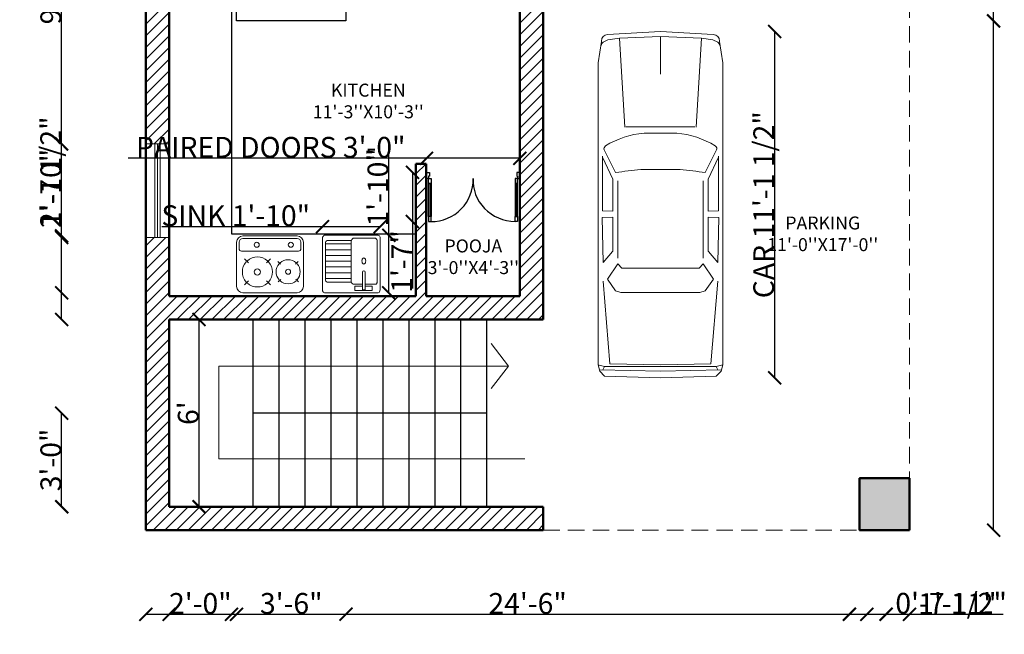
# Model space of a CAD drawing. Units: inches. Extents: x 1385 to 1778, y 1343 to 2100.
# Tile 1 of 6: x 1385 to 1764, y 1343 to 1579. Entities that reach past the tile are written whole.
import ezdxf

# ---------------------------------------------------------------- set-up
doc = ezdxf.new("R2010")
doc.units = ezdxf.units.IN
doc.linetypes.add('HIDDEN', pattern=[9.525, 6.35, -3.175])
for name, color, linetype, lineweight in [('A-ANNO-DIMS', 2, 'Continuous', 18), ('A-ANNO-SYMB', 50, 'Continuous', 18), ('A-AREA-IDEN', 7, 'Continuous', 25), ('A-COLS', 10, 'Continuous', 50), ('A-COLS-PATT', 10, 'Continuous', 13), ('A-EQPM', 9, 'Continuous', 18), ('A-FLOR-FIXT', 9, 'Continuous', 18), ('A-SITE-VEHI', 8, 'Continuous', 18), ('A-WALL-HIDN', 7, 'HIDDEN', 18), ('A-WALL-PATT', 8, 'Continuous', 13), ('Door', 150, 'Continuous', 25), ('Kitchen', 142, 'Continuous', 25), ('Steps', 50, 'Continuous', 25), ('Wall', 7, 'Continuous', 50), ('Windows', 140, 'Continuous', 18)]:
    doc.layers.add(name, color=color, linetype=linetype, lineweight=lineweight)
doc.layers.add('A-Glaz', color=92, linetype='Continuous')
doc.styles.get("Standard").update_dxf_attribs({"font": 'arial.ttf'})
doc.dimstyles.get("Standard").update_dxf_attribs({"dimtxt": 8, "dimasz": 5, "dimexe": 0.18, "dimexo": 0.0625, "dimgap": 0.09, "dimtad": 1, "dimdec": 1, "dimzin": 0, "dimdsep": 46, "dimlunit": 4, "dimtxsty": 'Standard', "dimblk": 'ARCHTICK', "dimcen": 0.09, "dimse1": 1, "dimse2": 1, "dimadec": 0, "dimazin": 0, "dimtfac": 1, "dimtdec": 1, "dimtofl": 0, "dimtmove": 0, "dimatfit": 3, "dimfxl": 1, "dimtolj": 1, "dimtzin": 0, "dimarcsym": 0})

# ---------------------------------------------------------------- blocks, each defined once
blk = doc.blocks.new('A$C13CE0A17')
at = {"layer": 'A-Glaz'}
for p, q in [((0.01, 0.61), (0.01, 0.08)), ((0.03, 0.08), (0.03, 0.61))]:
    blk.add_line(p, q, dxfattribs=at)
blk.add_lwpolyline([(1.4, 0.08), (1.4, 0.61), (1.42, 0.61), (1.42, 0.08)], close=True, dxfattribs=at)
at = {"layer": 'Door'}
for p, q in [((0, 0.61), (0, 0.69)), ((0, 0.69), (0.04, 0.69)), ((0.04, 0.69), (0.04, 0.61)), ((0, 0.61), (0, 0.08)), ((0.04, 0.61), (0, 0.61)), ((0.04, 0.61), (0, 0.61)), ((0.03, 0.61), (0.01, 0.61)), ((0.04, 0.08), (0.04, 0.61)), ((-0.035, 0), (-0.035, -0.1)), ((0, 0), (-0.035, 0)), ((0, 0.08), (0, 0)), ((0.04, 0.08), (0, 0.08)), ((0, 0.08), (0.04, 0.08)), ((0, 0), (0.04, 0)), ((0, -0.04), (0, 0)), ((0.01, 0.08), (0.03, 0.08)), ((0.04, 0), (0.04, 0.08)), ((-0.035, -0.1), (0.015, -0.1)), ((0.015, -0.04), (0, -0.04)), ((0.015, -0.05), (0.015, -0.04)), ((0.015, -0.1), (0.015, -0.05))]:
    blk.add_line(p, q, dxfattribs=at)
for points in [[(1.39, 0.69), (1.39, 0.61), (1.43, 0.61), (1.43, 0.69)], [(1.39, 0.08), (1.39, 0.61), (1.43, 0.61), (1.43, 0.08)], [(1.39, 0), (1.39, 0.08), (1.43, 0.08), (1.43, 0)], [(1.43, 0), (1.465, 0), (1.465, -0.1), (1.415, -0.1), (1.415, -0.05), (1.415, -0.04), (1.43, -0.04)]]:
    blk.add_lwpolyline(points, close=True, dxfattribs=at)
blk.add_arc((1.387, 0.017), 0.673, 89.7657, 181.4438, dxfattribs=at)
blk.add_ellipse((0.039, 0.051), major_axis=(0.667, -0.122), ratio=0.940794, start_param=0.11153, end_param=1.73917, dxfattribs=at)
blk = doc.blocks.new('02PCAR12')
at = {"color": 0, "linetype": 'ByBlock'}
for p, q in [((-207, 37), (-210, 34)), ((-203, 38), (-207, 37)), ((-206, 37), (-207, 0)), ((-203, 38.08), (-204, 34.08)), ((-19, 38), (-203, 38)), ((-6, 36), (-19, 38)), ((-210, 34), (-211, 0)), ((-204, 34.08), (-206, 35.08)), ((-204, -34), (-204, 34)), ((-202.36, 30.78), (-203, 0)), ((-202.36, 30.78), (-152, 35)), ((-150.83, 32.3), (-157.9, 27.3)), ((-141.48, 25.99), (-150.83, 32.3)), ((-113.23, 35.5), (-140.79, 34.89)), ((-140.79, 34.89), (-133.96, 29.23)), ((-113, 29), (-113.23, 35.5)), ((-109.42, 29.02), (-109.19, 35.33)), ((-109.19, 35.33), (-75.91, 35.3)), ((-76.45, 35.3), (-90, 29)), ((-72.15, 34.24), (-85.91, 27.37)), ((-5, 32), (-6.45, 34.89)), ((-5, 32), (-4, 25)), ((0, 0), (-1.8, 32.21)), ((-157.9, 27.3), (-158.93, 24.08)), ((-158.93, 24.08), (-158.93, -24)), ((-141.48, 25.99), (-144.24, 23.52)), ((-91, 26), (-138, 26)), ((-134, 29), (-113, 29)), ((-90, 29), (-109.42, 29.02)), ((-58.25, 21.76), (-4, 25)), ((-4, 25), (-3, 0)), ((-144.24, 23.52), (-144.24, 0)), ((-58, 0), (-58, 21)), ((-84, -12), (-84, 12)), ((-62, 10), (-62, 0)), ((-210, -34), (-211, 0)), ((-206, -37), (-207, 0)), ((-202.36, -30.78), (-203, 0)), ((-144.24, -23.52), (-144.24, 0)), ((-62, -10), (-62, 0)), ((-58, 0), (-58, -21)), ((-3, 0), (-26, 0)), ((-4, -25), (-3, 0)), ((0, 0), (-1.8, -32.21)), ((-141.48, -25.99), (-144.24, -23.52)), ((-58.25, -21.76), (-4, -25)), ((-157.9, -27.3), (-158.93, -24.08)), ((-150.83, -32.3), (-157.9, -27.3)), ((-141.48, -25.99), (-150.83, -32.3)), ((-140.79, -34.89), (-133.96, -29.23)), ((-91, -26), (-138, -26)), ((-134, -29), (-113, -29)), ((-113, -29), (-113.23, -35.5)), ((-90, -29), (-109.42, -29.02)), ((-109.42, -29.02), (-109.19, -35.33)), ((-76.45, -35.3), (-90, -29)), ((-72.15, -34.24), (-85.91, -27.37)), ((-5, -32), (-4, -25)), ((-207, -37), (-210, -34)), ((-204, -34), (-206, -35)), ((-203, -38), (-204, -34)), ((-202.36, -30.69), (-152, -34.92)), ((-113.23, -35.5), (-140.79, -34.89)), ((-109.19, -35.33), (-75.91, -35.3)), ((-6, -36), (-19, -38)), ((-5, -32), (-6.45, -34.89)), ((-203, -38), (-207, -37)), ((-19, -38), (-203, -38))]:
    blk.add_line(p, q, dxfattribs=at)
for centre, radius, start, end in [((-71.36, 32.4), 2, 31.5638, 113.12574), ((-115.33, 5.39), 53.61, 4.93792, 31.5638), ((-8.24, 34), 2, 26.56505, 90), ((-5.8, 32), 4, 3.01279, 90), ((-461.05, -27.14), 379.08, 5.92644, 8.26698), ((-461.05, 27.14), 379.08, 351.73302, 354.07356), ((-115.33, -5.39), 53.61, 328.4362, 355.06208), ((-71.36, -32.4), 2, 246.87426, 328.4362), ((-8.24, -34), 2, 270, 333.43495), ((-5.8, -32), 4, 270, 356.98721)]:
    blk.add_arc(centre, radius, start, end, dxfattribs=at)
blk = doc.blocks.new('S_SINK12')
for p, q in [((0.25, 0.45), (0.25, 0)), ((0.35, 0.45), (0.35, 0)), ((0.45, 0.45), (0.45, 0)), ((0.55, 0.45), (0.55, 0)), ((0.65, 0.45), (0.65, 0)), ((0.75, 0.45), (0.75, 0)), ((0.85, 0.45), (0.85, 0))]:
    blk.add_line(p, q)
for points in [[(0, -0.469), (0, 0.469, -0.310961), (0.05, 0.5), (0.95, 0.5, -0.310466), (1, 0.469), (1, -0.469, -0.414214), (0.969, -0.5), (0.05, -0.5, -0.309971)], [(0.052, -0.195), (0.052, -0.242), (0.362, -0.242, 1), (0.362, -0.195)], [(0.5, -0.217), (0.503, -0.229, 0.107136), (0.516, -0.241, 0.076468), (0.534, -0.249), (0.554, -0.251), (0.575, -0.248, 0.076468), (0.592, -0.241, 0.107136), (0.604, -0.229), (0.608, -0.217), (0.604, -0.205, 0.107136), (0.592, -0.193, 0.076468), (0.575, -0.186), (0.554, -0.183), (0.532, -0.186, 0.076468), (0.516, -0.193, 0.107136), (0.503, -0.205)]]:
    blk.add_lwpolyline(points, format="xyb", close=True)
for points in [[(0.185, -0.001), (0.185, 0.419, -0.310466), (0.235, 0.45), (0.862, 0.45, -0.310466), (0.912, 0.419), (0.912, 0, -0.310466)], [(0.15, -0.195), (0.15, -0.031, -0.310466), (0.2, 0), (0.9, 0, -0.310466), (0.95, -0.031), (0.95, -0.419, -0.310466), (0.9, -0.45), (0.2, -0.45), (0.18, -0.448, -0.071009), (0.165, -0.442, -0.106323), (0.153, -0.432), (0.15, -0.422), (0.151, -0.419)]]:
    blk.add_lwpolyline(points, format="xyb")
for points in [[(0.114, -0.242), (0.114, -0.364), (0.039, -0.364), (0.039, -0.064), (0.114, -0.064), (0.114, -0.195)], [(0.15, -0.419), (0.15, -0.242)]]:
    blk.add_lwpolyline(points)
blk = doc.blocks.new('_ArchTick')
at = {"color": 0, "linetype": 'ByBlock', "const_width": 0.15}
blk.add_lwpolyline([(-0.5, -0.5), (0.5, 0.5)], dxfattribs=at)
blk = doc.blocks.new('*D12')
at = {"layer": 'A-ANNO-DIMS', "color": 0, "lineweight": -2, "transparency": 16777216}
blk.add_line((1454.26, 1391.73), (1454.26, 1463.73), dxfattribs=at)
at = {"layer": 'Defpoints', "color": 0, "transparency": 16777216}
for p in [(1442.77, 1463.73), (1454.26, 1463.73), (1442.77, 1391.73)]:
    blk.add_point(p, dxfattribs=at)
at = {"layer": 'A-ANNO-DIMS', "color": 0, "lineweight": -2, "transparency": 16777216, "xscale": 5, "yscale": 5, "zscale": 5}
for p, rotation in [((1454.26, 1463.73), 90), ((1454.26, 1391.73), 270)]:
    blk.add_blockref('_ArchTick', p, dxfattribs=dict(at, rotation=rotation))
at = {"layer": 'A-ANNO-DIMS', "color": 0, "transparency": 16777216, "insert": (1450.09, 1427.73), "char_height": 8, "attachment_point": 5, "rotation": 90}
blk.add_mtext("\\A1;6'", dxfattribs=at)
blk = doc.blocks.new('WINDOW-GLAZING-36IN')
for p, q in [((0, 0), (0, 36)), ((1, 0), (1, 36)), ((2, 0), (2, 36))]:
    blk.add_line(p, q)
blk = doc.blocks.new('*D25')
at = {"layer": 'A-ANNO-DIMS', "color": 0, "lineweight": -2, "transparency": 16777216}
for p, q in [((1541.8, 1525.8), (1426.95, 1525.8)), ((1577.76, 1525.8), (1541.8, 1525.8))]:
    blk.add_line(p, q, dxfattribs=at)
at = {"layer": 'Defpoints', "color": 0, "transparency": 16777216}
for p in [(1541.8, 1525.8), (1541.8, 1520.41), (1577.76, 1520.41)]:
    blk.add_point(p, dxfattribs=at)
at = {"layer": 'A-ANNO-DIMS', "color": 0, "lineweight": -2, "transparency": 16777216, "xscale": 5, "yscale": 5, "zscale": 5, "rotation": 180}
blk.add_blockref('_ArchTick', (1541.8, 1525.8), dxfattribs=at)
at = {"layer": 'A-ANNO-DIMS', "color": 0, "lineweight": -2, "transparency": 16777216, "xscale": 5, "yscale": 5, "zscale": 5}
blk.add_blockref('_ArchTick', (1577.76, 1525.8), dxfattribs=at)
at = {"layer": 'A-ANNO-DIMS', "color": 0, "transparency": 16777216, "insert": (1481.87, 1530.04), "char_height": 8, "attachment_point": 5}
blk.add_mtext('\\A1;PAIRED DOORS 3\'-0"', dxfattribs=at)
blk = doc.blocks.new('*D26')
at = {"layer": 'A-ANNO-DIMS', "color": 0, "lineweight": -2, "transparency": 16777216}
for p, q in [((1536.41, 1520.41), (1536.41, 1501.46)), ((1536.41, 1501.46), (1536.41, 1475.76))]:
    blk.add_line(p, q, dxfattribs=at)
at = {"layer": 'Defpoints', "color": 0, "transparency": 16777216}
for p in [(1541.8, 1520.41), (1536.41, 1501.46), (1541.8, 1501.46)]:
    blk.add_point(p, dxfattribs=at)
at = {"layer": 'A-ANNO-DIMS', "color": 0, "lineweight": -2, "transparency": 16777216, "xscale": 5, "yscale": 5, "zscale": 5}
for p, rotation in [((1536.41, 1520.41), 90), ((1536.41, 1501.46), 270)]:
    blk.add_blockref('_ArchTick', p, dxfattribs=dict(at, rotation=rotation))
at = {"layer": 'A-ANNO-DIMS', "color": 0, "transparency": 16777216, "insert": (1532.3, 1486.11), "char_height": 8, "attachment_point": 5, "rotation": 90}
blk.add_mtext('\\A1;1\'-7"', dxfattribs=at)
blk = doc.blocks.new('*D39')
at = {"layer": 'A-ANNO-DIMS', "color": 0, "lineweight": -2, "transparency": 16777216}
blk.add_line((1675.9, 1441.31), (1675.9, 1574.58), dxfattribs=at)
at = {"layer": 'Defpoints', "color": 0, "transparency": 16777216}
for p in [(1655.9, 1574.58), (1675.9, 1574.58), (1655.9, 1441.31)]:
    blk.add_point(p, dxfattribs=at)
at = {"layer": 'A-ANNO-DIMS', "color": 0, "lineweight": -2, "transparency": 16777216, "xscale": 5, "yscale": 5, "zscale": 5}
for p, rotation in [((1675.9, 1574.58), 90), ((1675.9, 1441.31), 270)]:
    blk.add_blockref('_ArchTick', p, dxfattribs=dict(at, rotation=rotation))
at = {"layer": 'A-ANNO-DIMS', "color": 0, "transparency": 16777216, "insert": (1671.67, 1507.94), "char_height": 8, "attachment_point": 5, "rotation": 90}
blk.add_mtext('\\A1;CAR 11\'-1 1/2"', dxfattribs=at)
blk = doc.blocks.new('*D40')
at = {"layer": 'A-ANNO-DIMS', "color": 0, "lineweight": -2, "transparency": 16777216}
blk.add_line((1655.9, 1594.57), (1607.85, 1594.57), dxfattribs=at)
at = {"layer": 'Defpoints', "color": 0, "transparency": 16777216}
for p in [(1607.85, 1594.57), (1607.85, 1574.58), (1655.9, 1574.58)]:
    blk.add_point(p, dxfattribs=at)
at = {"layer": 'A-ANNO-DIMS', "color": 0, "lineweight": -2, "transparency": 16777216, "xscale": 5, "yscale": 5, "zscale": 5, "rotation": 180}
blk.add_blockref('_ArchTick', (1607.85, 1594.57), dxfattribs=at)
at = {"layer": 'A-ANNO-DIMS', "color": 0, "lineweight": -2, "transparency": 16777216, "xscale": 5, "yscale": 5, "zscale": 5}
blk.add_blockref('_ArchTick', (1655.9, 1594.57), dxfattribs=at)
at = {"layer": 'A-ANNO-DIMS', "color": 0, "transparency": 16777216, "insert": (1631.88, 1598.75), "char_height": 8, "attachment_point": 5}
blk.add_mtext('\\A1;4\'-0"', dxfattribs=at)
blk = doc.blocks.new('*D43')
at = {"layer": 'A-ANNO-DIMS', "color": 0, "lineweight": -2, "transparency": 16777216}
for p, q in [((1501.79, 1499.49), (1439.98, 1499.49)), ((1523.98, 1499.49), (1501.79, 1499.49))]:
    blk.add_line(p, q, dxfattribs=at)
at = {"layer": 'Defpoints', "color": 0, "transparency": 16777216}
for p in [(1501.79, 1499.49), (1501.79, 1496.16), (1523.98, 1496.16)]:
    blk.add_point(p, dxfattribs=at)
at = {"layer": 'A-ANNO-DIMS', "color": 0, "lineweight": -2, "transparency": 16777216, "xscale": 5, "yscale": 5, "zscale": 5, "rotation": 180}
blk.add_blockref('_ArchTick', (1501.79, 1499.49), dxfattribs=at)
at = {"layer": 'A-ANNO-DIMS', "color": 0, "lineweight": -2, "transparency": 16777216, "xscale": 5, "yscale": 5, "zscale": 5}
blk.add_blockref('_ArchTick', (1523.98, 1499.49), dxfattribs=at)
at = {"layer": 'A-ANNO-DIMS', "color": 0, "transparency": 16777216, "insert": (1468.39, 1503.72), "char_height": 8, "attachment_point": 5}
blk.add_mtext('\\A1;SINK 1\'-10"', dxfattribs=at)
blk = doc.blocks.new('*D44')
at = {"layer": 'A-ANNO-DIMS', "color": 0, "lineweight": -2, "transparency": 16777216}
for p, q in [((1527.31, 1496.16), (1527.31, 1528.07)), ((1527.31, 1474.02), (1527.31, 1496.16))]:
    blk.add_line(p, q, dxfattribs=at)
at = {"layer": 'Defpoints', "color": 0, "transparency": 16777216}
for p in [(1523.98, 1496.16), (1527.31, 1496.16), (1523.98, 1474.02)]:
    blk.add_point(p, dxfattribs=at)
at = {"layer": 'A-ANNO-DIMS', "color": 0, "lineweight": -2, "transparency": 16777216, "xscale": 5, "yscale": 5, "zscale": 5}
for p, rotation in [((1527.31, 1496.16), 90), ((1527.31, 1474.02), 270)]:
    blk.add_blockref('_ArchTick', p, dxfattribs=dict(at, rotation=rotation))
at = {"layer": 'A-ANNO-DIMS', "color": 0, "transparency": 16777216, "insert": (1523.13, 1514.62), "char_height": 8, "attachment_point": 5, "rotation": 90}
blk.add_mtext('\\A1;1\'-10"', dxfattribs=at)
blk = doc.blocks.new('*D49')
at = {"layer": 'A-ANNO-DIMS', "color": 0, "lineweight": -2, "transparency": 16777216}
blk.add_line((1433.77, 1350.33), (1727.77, 1350.33), dxfattribs=at)
at = {"layer": 'Defpoints', "color": 0, "transparency": 16777216}
for p in [(1433.77, 1382.73), (1727.77, 1382.73), (1727.77, 1350.33)]:
    blk.add_point(p, dxfattribs=at)
at = {"layer": 'A-ANNO-DIMS', "color": 0, "lineweight": -2, "transparency": 16777216, "xscale": 5, "yscale": 5, "zscale": 5, "rotation": 180}
blk.add_blockref('_ArchTick', (1433.77, 1350.33), dxfattribs=at)
at = {"layer": 'A-ANNO-DIMS', "color": 0, "lineweight": -2, "transparency": 16777216, "xscale": 5, "yscale": 5, "zscale": 5}
blk.add_blockref('_ArchTick', (1727.77, 1350.33), dxfattribs=at)
at = {"layer": 'A-ANNO-DIMS', "color": 0, "transparency": 16777216, "insert": (1580.77, 1354.5), "char_height": 8, "attachment_point": 5}
blk.add_mtext('\\A1;24\'-6"', dxfattribs=at)
blk = doc.blocks.new('*D50')
at = {"layer": 'A-ANNO-DIMS', "color": 0, "lineweight": -2, "transparency": 16777216}
blk.add_line((1760.18, 1382.73), (1760.18, 2030.73), dxfattribs=at)
at = {"layer": 'Defpoints', "color": 0, "transparency": 16777216}
for p in [(1727.77, 2030.73), (1760.18, 2030.73), (1727.77, 1382.73)]:
    blk.add_point(p, dxfattribs=at)
at = {"layer": 'A-ANNO-DIMS', "color": 0, "lineweight": -2, "transparency": 16777216, "xscale": 5, "yscale": 5, "zscale": 5}
for p, rotation in [((1760.18, 2030.73), 90), ((1760.18, 1382.73), 270)]:
    blk.add_blockref('_ArchTick', p, dxfattribs=dict(at, rotation=rotation))
at = {"layer": 'A-ANNO-DIMS', "color": 0, "transparency": 16777216, "insert": (1756, 1706.73), "char_height": 8, "attachment_point": 5, "rotation": 90}
blk.add_mtext('\\A1;54\'-0"', dxfattribs=at)
blk = doc.blocks.new('*D59')
at = {"layer": 'A-ANNO-DIMS', "color": 0, "lineweight": -2, "transparency": 16777216}
blk.add_line((1401.37, 1531.33), (1401.37, 1647.46), dxfattribs=at)
at = {"layer": 'Defpoints', "color": 0, "transparency": 16777216}
for p in [(1401.37, 1647.46), (1433.77, 1647.46), (1433.77, 1531.33)]:
    blk.add_point(p, dxfattribs=at)
at = {"layer": 'A-ANNO-DIMS', "color": 0, "lineweight": -2, "transparency": 16777216, "xscale": 5, "yscale": 5, "zscale": 5}
for p, rotation in [((1401.37, 1647.46), 90), ((1401.37, 1531.33), 270)]:
    blk.add_blockref('_ArchTick', p, dxfattribs=dict(at, rotation=rotation))
at = {"layer": 'A-ANNO-DIMS', "color": 0, "transparency": 16777216, "insert": (1397.19, 1589.39), "char_height": 8, "attachment_point": 5, "rotation": 90}
blk.add_mtext('\\A1;9\'-8"', dxfattribs=at)
blk = doc.blocks.new('*D60')
at = {"layer": 'A-ANNO-DIMS', "color": 0, "lineweight": -2, "transparency": 16777216}
for p, q in [((1401.37, 1495.33), (1401.37, 1540.55)), ((1401.37, 1463.73), (1401.37, 1495.33))]:
    blk.add_line(p, q, dxfattribs=at)
at = {"layer": 'Defpoints', "color": 0, "transparency": 16777216}
for p in [(1401.37, 1495.33), (1433.77, 1495.33), (1442.77, 1463.73)]:
    blk.add_point(p, dxfattribs=at)
at = {"layer": 'A-ANNO-DIMS', "color": 0, "lineweight": -2, "transparency": 16777216, "xscale": 5, "yscale": 5, "zscale": 5}
for p, rotation in [((1401.37, 1495.33), 90), ((1401.37, 1463.73), 270)]:
    blk.add_blockref('_ArchTick', p, dxfattribs=dict(at, rotation=rotation))
at = {"layer": 'A-ANNO-DIMS', "color": 0, "transparency": 16777216, "insert": (1397.14, 1520.44), "char_height": 8, "attachment_point": 5, "rotation": 90}
blk.add_mtext('\\A1;2\'-7 1/2"', dxfattribs=at)
blk = doc.blocks.new('*D61')
at = {"layer": 'A-ANNO-DIMS', "color": 0, "lineweight": -2, "transparency": 16777216}
blk.add_line((1586.77, 2063.14), (1708.55, 2063.14), dxfattribs=at)
at = {"layer": 'Defpoints', "color": 0, "transparency": 16777216}
for p in [(1708.55, 2063.14), (1586.77, 1382.73), (1708.55, 1382.73)]:
    blk.add_point(p, dxfattribs=at)
at = {"layer": 'A-ANNO-DIMS', "color": 0, "lineweight": -2, "transparency": 16777216, "xscale": 5, "yscale": 5, "zscale": 5, "rotation": 180}
blk.add_blockref('_ArchTick', (1586.77, 2063.14), dxfattribs=at)
at = {"layer": 'A-ANNO-DIMS', "color": 0, "lineweight": -2, "transparency": 16777216, "xscale": 5, "yscale": 5, "zscale": 5}
blk.add_blockref('_ArchTick', (1708.55, 2063.14), dxfattribs=at)
at = {"layer": 'A-ANNO-DIMS', "color": 0, "transparency": 16777216, "insert": (1647.66, 2067.31), "char_height": 8, "attachment_point": 5}
blk.add_mtext('\\A1;10\'-2"', dxfattribs=at)
blk = doc.blocks.new('*D62')
at = {"layer": 'A-ANNO-DIMS', "color": 0, "lineweight": -2, "transparency": 16777216}
for p, q in [((1442.77, 2063.14), (1475.11, 2063.14)), ((1475.11, 2063.14), (1520.34, 2063.14))]:
    blk.add_line(p, q, dxfattribs=at)
at = {"layer": 'Defpoints', "color": 0, "transparency": 16777216}
for p in [(1475.11, 2063.14), (1442.77, 1391.73), (1475.11, 1391.73)]:
    blk.add_point(p, dxfattribs=at)
at = {"layer": 'A-ANNO-DIMS', "color": 0, "lineweight": -2, "transparency": 16777216, "xscale": 5, "yscale": 5, "zscale": 5, "rotation": 180}
blk.add_blockref('_ArchTick', (1442.77, 2063.14), dxfattribs=at)
at = {"layer": 'A-ANNO-DIMS', "color": 0, "lineweight": -2, "transparency": 16777216, "xscale": 5, "yscale": 5, "zscale": 5}
blk.add_blockref('_ArchTick', (1475.11, 2063.14), dxfattribs=at)
at = {"layer": 'A-ANNO-DIMS', "color": 0, "transparency": 16777216, "insert": (1500.22, 2067.37), "char_height": 8, "attachment_point": 5}
blk.add_mtext('\\A1;2\'-8 1/2"', dxfattribs=at)
blk = doc.blocks.new('*D63')
at = {"layer": 'A-ANNO-DIMS', "color": 0, "lineweight": -2, "transparency": 16777216}
for p, q in [((1475.11, 2063.14), (1485.11, 2063.14)), ((1485.11, 2063.14), (1517.77, 2063.14))]:
    blk.add_line(p, q, dxfattribs=at)
at = {"layer": 'Defpoints', "color": 0, "transparency": 16777216}
for p in [(1485.11, 2063.14), (1475.11, 1391.73), (1485.11, 1391.73)]:
    blk.add_point(p, dxfattribs=at)
at = {"layer": 'A-ANNO-DIMS', "color": 0, "lineweight": -2, "transparency": 16777216, "xscale": 5, "yscale": 5, "zscale": 5, "rotation": 180}
blk.add_blockref('_ArchTick', (1475.11, 2063.14), dxfattribs=at)
at = {"layer": 'A-ANNO-DIMS', "color": 0, "lineweight": -2, "transparency": 16777216, "xscale": 5, "yscale": 5, "zscale": 5}
blk.add_blockref('_ArchTick', (1485.11, 2063.14), dxfattribs=at)
at = {"layer": 'A-ANNO-DIMS', "color": 0, "transparency": 16777216, "insert": (1503.94, 2067.31), "char_height": 8, "attachment_point": 5}
blk.add_mtext('\\A1;0\'-10"', dxfattribs=at)
blk = doc.blocks.new('*D64')
at = {"layer": 'A-ANNO-DIMS', "color": 0, "lineweight": -2, "transparency": 16777216}
blk.add_line((1401.37, 1391.73), (1401.37, 1427.73), dxfattribs=at)
at = {"layer": 'Defpoints', "color": 0, "transparency": 16777216}
for p in [(1401.37, 1427.73), (1475.11, 1427.73), (1475.11, 1391.73)]:
    blk.add_point(p, dxfattribs=at)
at = {"layer": 'A-ANNO-DIMS', "color": 0, "lineweight": -2, "transparency": 16777216, "xscale": 5, "yscale": 5, "zscale": 5}
for p, rotation in [((1401.37, 1427.73), 90), ((1401.37, 1391.73), 270)]:
    blk.add_blockref('_ArchTick', p, dxfattribs=dict(at, rotation=rotation))
at = {"layer": 'A-ANNO-DIMS', "color": 0, "transparency": 16777216, "insert": (1397.19, 1409.73), "char_height": 8, "attachment_point": 5, "rotation": 90}
blk.add_mtext('\\A1;3\'-0"', dxfattribs=at)
blk = doc.blocks.new('*D65')
at = {"layer": 'A-ANNO-DIMS', "color": 0, "lineweight": -2, "transparency": 16777216}
blk.add_line((1442.77, 1350.33), (1466.77, 1350.33), dxfattribs=at)
at = {"layer": 'Defpoints', "color": 0, "transparency": 16777216}
for p in [(1442.77, 1595.73), (1466.77, 1595.73), (1466.77, 1350.33)]:
    blk.add_point(p, dxfattribs=at)
at = {"layer": 'A-ANNO-DIMS', "color": 0, "lineweight": -2, "transparency": 16777216, "xscale": 5, "yscale": 5, "zscale": 5, "rotation": 180}
blk.add_blockref('_ArchTick', (1442.77, 1350.33), dxfattribs=at)
at = {"layer": 'A-ANNO-DIMS', "color": 0, "lineweight": -2, "transparency": 16777216, "xscale": 5, "yscale": 5, "zscale": 5}
blk.add_blockref('_ArchTick', (1466.77, 1350.33), dxfattribs=at)
at = {"layer": 'A-ANNO-DIMS', "color": 0, "transparency": 16777216, "insert": (1454.77, 1354.5), "char_height": 8, "attachment_point": 5}
blk.add_mtext('\\A1;2\'-0"', dxfattribs=at)
blk = doc.blocks.new('*D68')
at = {"layer": 'A-ANNO-DIMS', "color": 0, "lineweight": -2, "transparency": 16777216}
for p, q in [((1704.65, 1350.33), (1727.77, 1350.33)), ((1727.77, 1350.33), (1759.68, 1350.33))]:
    blk.add_line(p, q, dxfattribs=at)
at = {"layer": 'Defpoints', "color": 0, "transparency": 16777216}
for p in [(1704.65, 1595.73), (1727.77, 1595.73), (1727.77, 1350.33)]:
    blk.add_point(p, dxfattribs=at)
at = {"layer": 'A-ANNO-DIMS', "color": 0, "lineweight": -2, "transparency": 16777216, "xscale": 5, "yscale": 5, "zscale": 5, "rotation": 180}
blk.add_blockref('_ArchTick', (1704.65, 1350.33), dxfattribs=at)
at = {"layer": 'A-ANNO-DIMS', "color": 0, "lineweight": -2, "transparency": 16777216, "xscale": 5, "yscale": 5, "zscale": 5}
blk.add_blockref('_ArchTick', (1727.77, 1350.33), dxfattribs=at)
at = {"layer": 'A-ANNO-DIMS', "color": 0, "transparency": 16777216, "insert": (1746.23, 1354.44), "char_height": 8, "attachment_point": 5}
blk.add_mtext('\\A1;1\'-11"', dxfattribs=at)
blk = doc.blocks.new('*D73')
at = {"layer": 'A-ANNO-DIMS', "color": 0, "lineweight": -2, "transparency": 16777216}
blk.add_line((1468.71, 2063.14), (1494.47, 2063.14), dxfattribs=at)
at = {"layer": 'Defpoints', "color": 0, "transparency": 16777216}
for p in [(1494.47, 2063.14), (1468.71, 1493.49), (1494.47, 1493.49)]:
    blk.add_point(p, dxfattribs=at)
at = {"layer": 'A-ANNO-DIMS', "color": 0, "lineweight": -2, "transparency": 16777216, "xscale": 5, "yscale": 5, "zscale": 5, "rotation": 180}
blk.add_blockref('_ArchTick', (1468.71, 2063.14), dxfattribs=at)
at = {"layer": 'A-ANNO-DIMS', "color": 0, "lineweight": -2, "transparency": 16777216, "xscale": 5, "yscale": 5, "zscale": 5}
blk.add_blockref('_ArchTick', (1494.47, 2063.14), dxfattribs=at)
at = {"layer": 'A-ANNO-DIMS', "color": 0, "transparency": 16777216, "insert": (1481.59, 2067.25), "char_height": 8, "attachment_point": 5}
blk.add_mtext('\\A1;2\'-2"', dxfattribs=at)
blk = doc.blocks.new('*D74')
at = {"layer": 'A-ANNO-DIMS', "color": 0, "lineweight": -2, "transparency": 16777216}
for p, q in [((1401.37, 1495.92), (1401.37, 1527.83)), ((1401.37, 1474.05), (1401.37, 1495.92))]:
    blk.add_line(p, q, dxfattribs=at)
at = {"layer": 'Defpoints', "color": 0, "transparency": 16777216}
for p in [(1401.37, 1495.92), (1471.14, 1495.92), (1471.14, 1474.05)]:
    blk.add_point(p, dxfattribs=at)
at = {"layer": 'A-ANNO-DIMS', "color": 0, "lineweight": -2, "transparency": 16777216, "xscale": 5, "yscale": 5, "zscale": 5}
for p, rotation in [((1401.37, 1495.92), 90), ((1401.37, 1474.05), 270)]:
    blk.add_blockref('_ArchTick', p, dxfattribs=dict(at, rotation=rotation))
at = {"layer": 'A-ANNO-DIMS', "color": 0, "transparency": 16777216, "insert": (1397.19, 1514.38), "char_height": 8, "attachment_point": 5, "rotation": 90}
blk.add_mtext('\\A1;1\'-10"', dxfattribs=at)
blk = doc.blocks.new('*D76')
at = {"layer": 'A-ANNO-DIMS', "color": 0, "lineweight": -2, "transparency": 16777216}
for p, q in [((1711.39, 1350.33), (1718.77, 1350.33)), ((1718.77, 1350.33), (1763.86, 1350.33))]:
    blk.add_line(p, q, dxfattribs=at)
at = {"layer": 'Defpoints', "color": 0, "transparency": 16777216}
for p in [(1711.39, 1970.73), (1718.77, 1970.73), (1718.77, 1350.33)]:
    blk.add_point(p, dxfattribs=at)
at = {"layer": 'A-ANNO-DIMS', "color": 0, "lineweight": -2, "transparency": 16777216, "xscale": 5, "yscale": 5, "zscale": 5, "rotation": 180}
blk.add_blockref('_ArchTick', (1711.39, 1350.33), dxfattribs=at)
at = {"layer": 'A-ANNO-DIMS', "color": 0, "lineweight": -2, "transparency": 16777216, "xscale": 5, "yscale": 5, "zscale": 5}
blk.add_blockref('_ArchTick', (1718.77, 1350.33), dxfattribs=at)
at = {"layer": 'A-ANNO-DIMS', "color": 0, "transparency": 16777216, "insert": (1743.82, 1354.56), "char_height": 8, "attachment_point": 5}
blk.add_mtext('\\A1;0\'-7 1/2"', dxfattribs=at)
blk = doc.blocks.new('*D80')
at = {"layer": 'A-ANNO-DIMS', "color": 0, "lineweight": -2, "transparency": 16777216}
blk.add_line((1468.72, 1350.33), (1510.83, 1350.33), dxfattribs=at)
at = {"layer": 'Defpoints', "color": 0, "transparency": 16777216}
for p in [(1468.72, 1578.65), (1510.83, 1578.65), (1510.83, 1350.33)]:
    blk.add_point(p, dxfattribs=at)
at = {"layer": 'A-ANNO-DIMS', "color": 0, "lineweight": -2, "transparency": 16777216, "xscale": 5, "yscale": 5, "zscale": 5, "rotation": 180}
blk.add_blockref('_ArchTick', (1468.72, 1350.33), dxfattribs=at)
at = {"layer": 'A-ANNO-DIMS', "color": 0, "lineweight": -2, "transparency": 16777216, "xscale": 5, "yscale": 5, "zscale": 5}
blk.add_blockref('_ArchTick', (1510.83, 1350.33), dxfattribs=at)
at = {"layer": 'A-ANNO-DIMS', "color": 0, "transparency": 16777216, "insert": (1489.77, 1354.51), "char_height": 8, "attachment_point": 5}
blk.add_mtext('\\A1;3\'-6"', dxfattribs=at)
blk = doc.blocks.new('*D81')
at = {"layer": 'A-ANNO-DIMS', "color": 0, "lineweight": -2, "transparency": 16777216}
for p, q in [((1760.18, 1591.85), (1760.18, 1617.54)), ((1760.18, 1578.65), (1760.18, 1591.85))]:
    blk.add_line(p, q, dxfattribs=at)
at = {"layer": 'Defpoints', "color": 0, "transparency": 16777216}
for p in [(1510.83, 1591.85), (1760.18, 1591.85), (1510.83, 1578.65)]:
    blk.add_point(p, dxfattribs=at)
at = {"layer": 'A-ANNO-DIMS', "color": 0, "lineweight": -2, "transparency": 16777216, "xscale": 5, "yscale": 5, "zscale": 5}
for p, rotation in [((1760.18, 1591.85), 90), ((1760.18, 1578.65), 270)]:
    blk.add_blockref('_ArchTick', p, dxfattribs=dict(at, rotation=rotation))
at = {"layer": 'A-ANNO-DIMS', "color": 0, "transparency": 16777216, "insert": (1756.07, 1607.19), "char_height": 8, "attachment_point": 5, "rotation": 90}
blk.add_mtext('\\A1;1\'-1"', dxfattribs=at)

msp = doc.modelspace()

# ---------------------------------------------------------------- hatches: boundary and pattern name
at = {"layer": 'A-COLS-PATT', "transparency": 33554585}
h = msp.add_hatch(color=256, dxfattribs=at)
h.dxf.hatch_style = 1
h.paths.add_polyline_path([(1727.77, 1402.71), (1708.55, 1402.71), (1708.55, 1382.73), (1727.77, 1382.73)])
at = {"layer": 'A-WALL-PATT', "transparency": 33554585}
h = msp.add_hatch(dxfattribs=at)
h.set_pattern_fill('ANSI31', color=256)
h.paths.add_polyline_path([(1522.75, 2030.73), (1433.77, 2030.73), (1433.77, 1900.6), (1442.77, 1900.6), (1442.77, 2021.73), (1522.75, 2021.73)])
h.paths.add_polyline_path([(1591.32, 2030.73), (1558.75, 2030.73), (1558.75, 2021.73), (1571.77, 2021.73), (1591.32, 2021.73)], flags=17)
h.paths.add_polyline_path([(1664.16, 2030.73), (1615.32, 2030.73), (1615.32, 2021.73), (1646.77, 2021.73), (1646.77, 1970.73), (1571.77, 1970.73), (1571.77, 1990.51, -0.048507), (1566.67, 1989.78), (1562.77, 1989.78), (1562.77, 1829.73), (1557.76, 1829.73), (1557.76, 1826.48), (1557.76, 1820.73), (1578.09, 1820.73), (1578.09, 1825.8), (1578.09, 1829.73), (1571.77, 1829.73), (1571.77, 1961.73), (1686.02, 1961.73), (1686.02, 1965.64, -0.048507), (1686.76, 1970.73), (1650.77, 1970.73), (1650.77, 2021.73), (1664.16, 2021.73)])
h.paths.add_polyline_path([(1727.77, 2030.73), (1688.16, 2030.73), (1688.16, 2021.73), (1718.77, 2021.73), (1718.77, 1970.73), (1711.39, 1970.73), (1711.39, 1965.64), (1711.39, 1961.73), (1718.77, 1961.73), (1718.77, 1904.94), (1727.77, 1904.94)])
h.paths.add_polyline_path([(1727.77, 1868.94), (1718.77, 1868.94), (1718.77, 1829.73), (1610.61, 1829.73, -0.028655), (1611.02, 1825.8), (1611.02, 1820.73), (1718.77, 1820.73), (1718.77, 1742.73), (1727.77, 1742.73)])
h.paths.add_polyline_path([(1520.45, 1826.48, -0.020905), (1520.74, 1829.73), (1442.77, 1829.73), (1442.77, 1840.6), (1433.77, 1840.6), (1433.77, 1794.33), (1442.77, 1794.33), (1442.77, 1820.73), (1502.77, 1820.73), (1502.77, 1760.73), (1497.07, 1760.73), (1497.07, 1759.8), (1497.07, 1754.73), (1508.77, 1754.73), (1508.77, 1778.73), (1562.77, 1778.73), (1562.77, 1656.82), (1571.77, 1656.82), (1571.77, 1784.73), (1508.77, 1784.73), (1508.77, 1820.73), (1520.45, 1820.73)])
h.paths.add_polyline_path([(1442.77, 1770.33), (1433.77, 1770.33), (1433.77, 1683.46), (1442.77, 1683.46)], flags=17)
h.paths.add_polyline_path([(1656.16, 1603.19, -0.007591), (1656.26, 1604.73), (1622.77, 1604.73), (1622.77, 1595.73), (1656.16, 1595.73)])
h.paths.add_polyline_path([(1727.77, 1682.73), (1718.77, 1682.73), (1718.77, 1604.73), (1704.65, 1604.73), (1704.65, 1603.19), (1704.65, 1595.73), (1727.77, 1595.73)])
h.paths.add_polyline_path([(1513.34, 1595.73), (1513.34, 1604.73), (1442.77, 1604.73), (1442.77, 1647.46), (1433.77, 1647.46), (1433.77, 1531.33), (1442.77, 1531.33), (1442.77, 1595.73)])
h.paths.add_polyline_path([(1546.08, 1604.73), (1546.08, 1595.73), (1577.77, 1595.73), (1577.77, 1472.73), (1541.77, 1472.73), (1541.77, 1523.73), (1537.77, 1523.73), (1537.77, 1472.73), (1442.77, 1472.73), (1442.77, 1495.33), (1433.77, 1495.33), (1433.77, 1382.73), (1586.77, 1382.73), (1586.77, 1391.73), (1442.77, 1391.73), (1442.77, 1463.73), (1586.77, 1463.73), (1586.77, 1604.73)])

# ---------------------------------------------------------------- linework, layer by layer
at = {"layer": 'A-ANNO-SYMB'}
for p, q in [((1573.41, 1445.86), (1566.68, 1454.56)), ((1461.82, 1410.21), (1461.82, 1445.86)), ((1461.82, 1445.86), (1573.41, 1445.86)), ((1573.41, 1445.86), (1566.68, 1437.17)), ((1579.69, 1410.21), (1461.82, 1410.21))]:
    msp.add_line(p, q, dxfattribs=at)
at = {"layer": 'A-COLS'}
msp.add_lwpolyline([(1727.77, 1382.73), (1708.55, 1382.73), (1708.55, 1402.71), (1727.77, 1402.71)], close=True, dxfattribs=at)
at = {"layer": 'A-EQPM'}
for p, q in [((1492.04, 1495.92), (1471.14, 1495.92)), ((1492.04, 1494.95), (1471.14, 1494.95)), ((1468.71, 1493.49), (1468.71, 1476.48)), ((1469.68, 1493.49), (1469.68, 1491.06)), ((1470.65, 1490.09), (1492.52, 1490.09)), ((1493.49, 1491.06), (1493.49, 1493.49)), ((1494.47, 1476.48), (1494.47, 1493.49)), ((1471.72, 1487.08), (1473.25, 1485.54)), ((1481.73, 1487.08), (1480.2, 1485.55)), ((1484.63, 1486.03), (1485.63, 1485.01)), ((1492.45, 1486.08), (1491.43, 1485.07)), ((1471.73, 1477.07), (1473.26, 1478.59)), ((1481.73, 1477.07), (1480.21, 1478.6)), ((1484.68, 1478.21), (1485.7, 1479.22)), ((1492.5, 1478.26), (1491.49, 1479.28)), ((1471.14, 1474.05), (1492.04, 1474.05))]:
    msp.add_line(p, q, dxfattribs=at)
for centre, radius in [((1476.48, 1492.52), 0.972), ((1489.61, 1492.52), 0.972), ((1476.73, 1482.07), 1.22), ((1488.56, 1482.14), 0.972)]:
    msp.add_circle(centre, radius, dxfattribs=at)
for centre, radius, start, end in [((1471.14, 1493.49), 2.43, 90, 180), ((1471.14, 1493.49), 1.46, 90, 180), ((1492.04, 1493.49), 2.43, 0, 90), ((1492.04, 1493.49), 1.46, 0, 90), ((1470.65, 1491.06), 0.972, 180, 270), ((1492.52, 1491.06), 0.972, 270, 0), ((1476.73, 1482.07), 5.79, 48.017, 131.983), ((1488.56, 1482.14), 4.62, 48.017, 131.983), ((1476.73, 1482.07), 5.79, 138.017, 221.983), ((1476.73, 1482.07), 5.79, 318.017, 41.983), ((1488.56, 1482.14), 4.62, 138.017, 221.983), ((1488.56, 1482.14), 4.62, 318.017, 41.983), ((1488.56, 1482.14), 4.62, 228.017, 311.983), ((1471.14, 1476.48), 2.43, 180, 270), ((1476.73, 1482.07), 5.79, 228.017, 311.983), ((1492.04, 1476.48), 2.43, 270, 0)]:
    msp.add_arc(centre, radius, start, end, dxfattribs=at)
at = {"layer": 'A-WALL-HIDN'}
for p in [(1727.77, 1595.73), (1586.77, 1382.73)]:
    msp.add_line(p, (1727.77, 1382.73), dxfattribs=at)
at = {"layer": 'Kitchen'}
for p, q in [((1466.77, 1595.73), (1466.77, 1496.73)), ((1466.77, 1496.73), (1537.77, 1496.73))]:
    msp.add_line(p, q, dxfattribs=at)
msp.add_lwpolyline([(1468.72, 1591.85), (1510.83, 1591.85), (1510.83, 1578.65), (1468.72, 1578.65)], close=True, dxfattribs=at)
at = {"layer": 'Steps'}
for p, q in [((1475.11, 1391.73), (1475.11, 1463.73)), ((1485.11, 1391.73), (1485.11, 1463.73)), ((1495.11, 1391.73), (1495.11, 1463.73)), ((1505.11, 1391.73), (1505.11, 1463.73)), ((1515.11, 1391.73), (1515.11, 1463.73)), ((1525.11, 1391.73), (1525.11, 1463.73)), ((1535.11, 1391.73), (1535.11, 1463.73)), ((1545.11, 1391.73), (1545.11, 1463.73)), ((1555.11, 1391.73), (1555.11, 1463.73)), ((1565.11, 1391.73), (1565.11, 1463.73)), ((1565.11, 1427.73), (1475.11, 1427.73))]:
    msp.add_line(p, q, dxfattribs=at)
at = {"layer": 'Wall'}
for p, q in [((1433.77, 2030.73), (1433.77, 1382.73)), ((1586.77, 1604.73), (1586.77, 1463.73)), ((1442.77, 1595.73), (1442.77, 1472.73)), ((1577.77, 1595.73), (1577.77, 1472.73)), ((1537.77, 1523.73), (1537.77, 1472.73)), ((1541.77, 1523.73), (1537.77, 1523.73)), ((1541.77, 1523.73), (1541.77, 1472.73)), ((1442.77, 1472.73), (1537.77, 1472.73)), ((1541.77, 1472.73), (1577.77, 1472.73)), ((1442.77, 1463.73), (1586.77, 1463.73)), ((1442.77, 1463.73), (1442.77, 1391.73)), ((1442.77, 1391.73), (1586.77, 1391.73)), ((1586.77, 1391.73), (1586.77, 1382.73)), ((1433.77, 1382.73), (1586.77, 1382.73))]:
    msp.add_line(p, q, dxfattribs=at)
at = {"layer": 'Windows'}
msp.add_lwpolyline([(1433.77, 1495.33), (1433.77, 1531.33), (1442.77, 1531.33), (1442.77, 1495.33)], close=True, dxfattribs=at)

# ---------------------------------------------------------------- block references
at = {"layer": 'A-FLOR-FIXT', "xscale": 22.14539759715611, "yscale": 22.14539759715611, "zscale": 22.14539759715611, "rotation": 90}
msp.add_blockref('S_SINK12', (1512.89, 1474.02), dxfattribs=at)
at = {"layer": 'A-SITE-VEHI', "xscale": 0.6316275775833333, "yscale": 0.6316275775833333, "zscale": 0.6316275775833333, "rotation": 90}
msp.add_blockref('02PCAR12', (1631.9, 1574.58), dxfattribs=at)
at = {"layer": 'Door', "xscale": 23.97117890612341, "yscale": 23.97117890612341, "zscale": 23.97117890612341, "rotation": 180}
msp.add_blockref('A$C13CE0A17', (1576.92, 1518.01), dxfattribs=at)
at = {"layer": 'Windows', "rotation": 180}
msp.add_blockref('WINDOW-GLAZING-36IN', (1439.27, 1531.33), dxfattribs=at)

# ---------------------------------------------------------------- texts
at = {"layer": 'A-AREA-IDEN', "char_height": 5, "attachment_point": 1}
for s, insert in [("\\pxqc;KITCHEN\\P11'-3''X10'-3''", (1494.28, 1554.53)), ("\\pxqc;PARKING\\P11'-0''X17'-0''", (1669.24, 1503.41)), ("\\pxqc;POOJA\\P3'-0''X4'-3''", (1534.72, 1494.58))]:
    msp.add_mtext_dynamic_manual_height_columns(s, width=50.3036, gutter_width=12.5, heights=[0], dxfattribs=dict(at, insert=insert))

# ---------------------------------------------------------------- dimensions: what is measured, and where the dimension line sits
at = {"layer": 'A-ANNO-DIMS'}
for base, p1, p2, picture, middle in [((1475.11, 2063.14), (1442.77, 1391.73), (1475.11, 1391.73), '*D62', (1500.22, 2067.37)), ((1494.47, 2063.14), (1468.71, 1493.49), (1494.47, 1493.49), '*D73', (1481.59, 2067.25)), ((1485.11, 2063.14), (1475.11, 1391.73), (1485.11, 1391.73), '*D63', (1503.94, 2067.31)), ((1708.55, 2063.14), (1586.77, 1382.73), (1708.55, 1382.73), '*D61', (1647.66, 2067.31)), ((1718.77, 1350.33), (1711.39, 1970.73), (1718.77, 1970.73), '*D76', (1743.82, 1354.56)), ((1466.77, 1350.33), (1442.77, 1595.73), (1466.77, 1595.73), '*D65', (1454.77, 1354.5)), ((1727.77, 1350.33), (1704.65, 1595.73), (1727.77, 1595.73), '*D68', (1746.23, 1354.44)), ((1510.83, 1350.33), (1468.72, 1578.65), (1510.83, 1578.65), '*D80', (1489.77, 1354.51)), ((1727.77, 1350.33), (1433.77, 1382.73), (1727.77, 1382.73), '*D49', (1580.77, 1354.5))]:
    dim = msp.add_linear_dim(base=base, p1=p1, p2=p2, dimstyle='Standard', override={"dimdec": 1, "dimlfac": 1, "dimrnd": 0, "dimzin": 1, "dimdsep": 46, "dimlunit": 4, "dimfrac": 2}, dxfattribs=at)
    dim.commit()
    dim.dimension.update_dxf_attribs({"geometry": picture, "text_midpoint": middle})
for base, p1, p2, angle, override, picture, middle in [((1760.18, 2030.73), (1727.77, 1382.73), (1727.77, 2030.73), 90, {"dimdec": 1, "dimlfac": 1, "dimrnd": 0, "dimzin": 1, "dimdsep": 46, "dimlunit": 4, "dimfrac": 2}, '*D50', (1756, 1706.73)), ((1401.37, 1647.46), (1433.77, 1531.33), (1433.77, 1647.46), 90, {"dimdec": 1, "dimlfac": 1, "dimrnd": 0, "dimzin": 1, "dimdsep": 46, "dimlunit": 4, "dimfrac": 2}, '*D59', (1397.19, 1589.39)), ((1760.18, 1591.85), (1510.83, 1578.65), (1510.83, 1591.85), 90, {"dimdec": 1, "dimlfac": 1, "dimrnd": 0, "dimzin": 1, "dimdsep": 46, "dimlunit": 4, "dimfrac": 2}, '*D81', (1756.07, 1607.19)), ((1607.8471, 1594.5714), (1655.904, 1574.5804), (1607.8471, 1574.5804), 180, {"dimdec": 1, "dimlfac": 1, "dimrnd": 0, "dimzin": 1, "dimdsep": 46, "dimlunit": 4, "dimfrac": 2}, '*D40', (1631.8756, 1598.746)), ((1401.37, 1495.33), (1442.77, 1463.73), (1433.77, 1495.33), 90, {"dimdec": 1, "dimlfac": 1, "dimrnd": 0, "dimzin": 1, "dimdsep": 46, "dimlunit": 4, "dimfrac": 2}, '*D60', (1397.14, 1520.44)), ((1401.37, 1495.92), (1471.14, 1474.05), (1471.14, 1495.92), 90, {"dimdec": 1, "dimlfac": 1, "dimrnd": 0, "dimzin": 1, "dimdsep": 46, "dimlunit": 4, "dimfrac": 2}, '*D74', (1397.19, 1514.38)), ((1527.31, 1496.16), (1523.98, 1474.02), (1523.98, 1496.16), 90, {"dimdec": 1, "dimlfac": 1, "dimrnd": 0, "dimzin": 1, "dimdsep": 46, "dimlunit": 4, "dimfrac": 2}, '*D44', (1523.13, 1514.62)), ((1536.4058, 1501.4559), (1541.7993, 1520.411), (1541.7993, 1501.4559), 270, {"dimdec": 1, "dimlfac": 1, "dimrnd": 0, "dimzin": 1, "dimdsep": 46, "dimlunit": 4, "dimfrac": 2}, '*D26', (1532.2994, 1486.1094)), ((1454.26, 1463.73), (1442.77, 1391.73), (1442.77, 1463.73), 90, {"dimclrd": 0, "dimclre": 0, "dimclrt": 0}, '*D12', (1450.09, 1427.73)), ((1401.37, 1427.73), (1475.11, 1391.73), (1475.11, 1427.73), 90, {"dimdec": 1, "dimlfac": 1, "dimrnd": 0, "dimzin": 1, "dimdsep": 46, "dimlunit": 4, "dimfrac": 2}, '*D64', (1397.19, 1409.73))]:
    dim = msp.add_linear_dim(base=base, p1=p1, p2=p2, angle=angle, dimstyle='Standard', override=override, dxfattribs=at)
    dim.commit()
    dim.dimension.update_dxf_attribs({"geometry": picture, "text_midpoint": middle})
for base, p1, p2, angle, text, picture, middle in [((1675.9, 1574.58), (1655.9, 1441.31), (1655.9, 1574.58), 90, 'CAR <>', '*D39', (1671.67, 1507.94)), ((1541.8, 1525.8), (1577.76, 1520.41), (1541.8, 1520.41), 180, 'PAIRED DOORS <>', '*D25', (1481.87, 1530.04)), ((1501.79, 1499.49), (1523.98, 1496.16), (1501.79, 1496.16), 180, 'SINK <>', '*D43', (1468.39, 1503.72))]:
    dim = msp.add_linear_dim(base=base, p1=p1, p2=p2, angle=angle, text=text, dimstyle='Standard', override={"dimdec": 1, "dimlfac": 1, "dimrnd": 0, "dimzin": 1, "dimdsep": 46, "dimlunit": 4, "dimfrac": 2}, dxfattribs=at)
    dim.commit()
    dim.dimension.update_dxf_attribs({"geometry": picture, "text_midpoint": middle})

doc.saveas('drawing.dxf')
